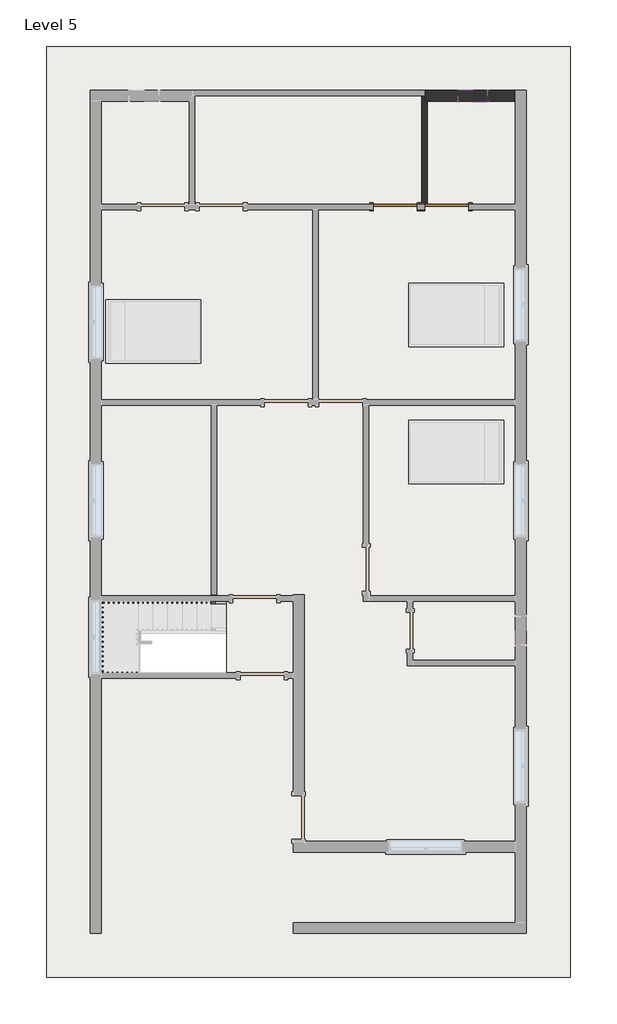
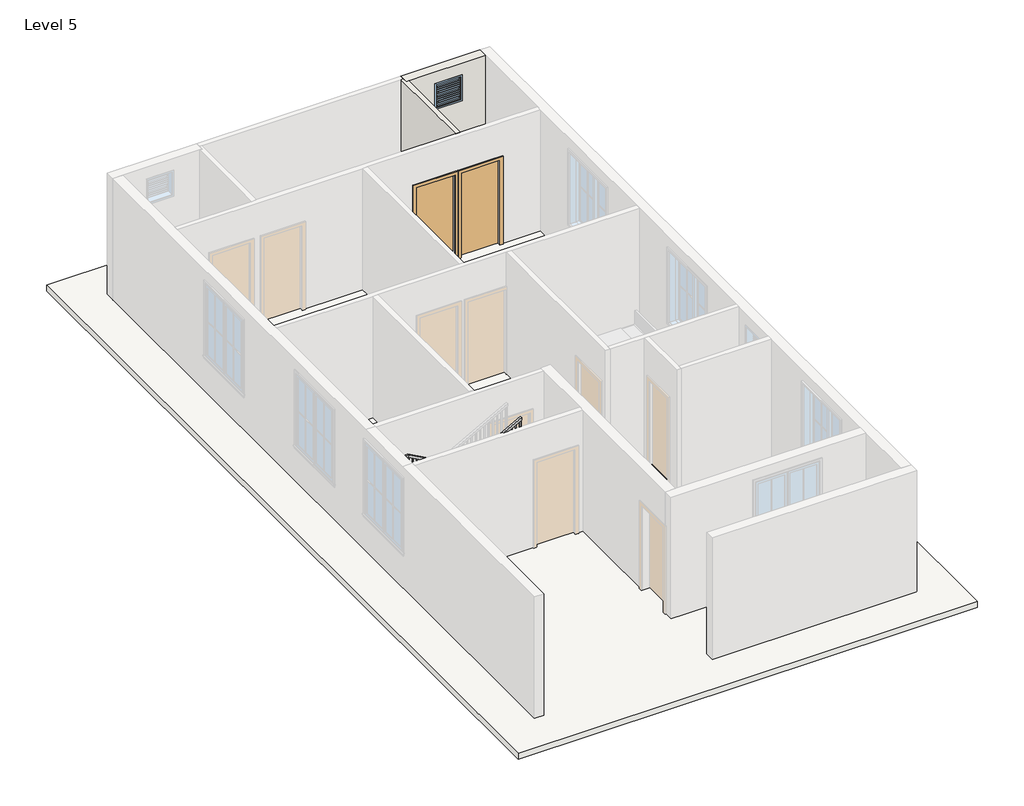
# One storey, part 2 of 3: 2 doors, 2 walls, 1 railing, 1 roof, 1 window.
"""IFC4 building model written with IfcOpenShell, lengths in millimetres."""

from ifc_helpers import new_model, si_unit, frame, origin, place, context, project, spatial, polyline, outline, extrude, faceted_brep, transform, mapped, element, save
from components import single_flush_door_3_e5f9f3c4, single_flush_door_3_305aa2a5, window_f2d8fef0

model = new_model("IFC4")

# Units and contexts
model_context = context("Model", 3, world=origin())
ifc_project = project(units=[si_unit("LENGTHUNIT", "METRE", prefix="MILLI")], contexts=[model_context])

# Site, building, storey
site = spatial("IfcSite", under=ifc_project)
building = spatial("IfcBuilding", under=site)
storey = spatial("IfcBuildingStorey", under=building, Name="Level 5", Elevation=9601.2)

# Doors
placement = place(None, origin())
single_flush_door_3_shape = single_flush_door_3_e5f9f3c4(model_context)
element("IfcDoor", 1, ObjectType="Single-Flush : DOOR 3'", at=placement, inside=storey, context=model_context, shape_type="MappedRepresentation", body=[
    mapped(single_flush_door_3_shape, transform((555.4379845, 6040.5434309, 9601.2), x_axis=(1.0, 0.0, 0.0), y_axis=(0.0, 1.0, 0.0), z_axis=(0.0, 0.0, 1.0))),
])
single_flush_door_3_2_shape = single_flush_door_3_305aa2a5(model_context)
element("IfcDoor", 2, ObjectType="Single-Flush : DOOR 3'", at=placement, inside=storey, context=model_context, shape_type="MappedRepresentation", body=[
    mapped(single_flush_door_3_2_shape, transform((1622.2379845, 6040.5434309, 9601.2), x_axis=(-1.0, 0.0, 0.0), y_axis=(0.0, -1.0, 0.0), z_axis=(0.0, 0.0, 1.0))),
])

# Railing
element("IfcRailing", 3, ObjectType="Handrail - Rectangular", at=placement, inside=storey, context=model_context, shape_type="SolidModel", body=[
    faceted_brep([(-2968.8120155, -2220.8065691, 10684.9333333), (-2968.8120155, -2220.8065691, 10626.820221), (-2968.8120155, -2170.0065691, 10626.820221), (-2968.8120155, -2170.0065691, 10684.9333333), (-4797.6120155, -2220.8065691, 11700.9333333), (-4810.7756177, -2220.8065691, 11650.1333333), (-4810.7756177, -2170.0065691, 11650.1333333), (-4797.6120155, -2170.0065691, 11700.9333333), (-5508.8120155, -2220.8065691, 11700.9333333), (-5508.8120155, -2220.8065691, 11650.1333333), (-5559.6120155, -2170.0065691, 11650.1333333), (-5559.6120155, -2170.0065691, 11700.9333333), (-5508.8120155, -3624.1565691, 11700.9333333), (-5508.8120155, -3624.1565691, 11650.1333333), (-5559.6120155, -3674.9565691, 11650.1333333), (-5559.6120155, -3674.9565691, 11700.9333333), (-5102.4120155, -3624.1565691, 11700.9333333), (-5089.2484132, -3624.1565691, 11650.1333333), (-5089.2484132, -3674.9565691, 11650.1333333), (-5102.4120155, -3674.9565691, 11700.9333333), (-2968.8120155, -3624.1565691, 12886.2666667), (-2968.8120155, -3674.9565691, 12886.2666667), (-2968.8120155, -3674.9565691, 12828.1535543), (-2968.8120155, -3624.1565691, 12828.1535543)], [[[0, 1, 2, 3]], [[1, 0, 4, 5]], [[2, 1, 5, 6]], [[3, 2, 6, 7]], [[0, 3, 7, 4]], [[5, 4, 8, 9]], [[6, 5, 9, 10]], [[7, 6, 10, 11]], [[4, 7, 11, 8]], [[9, 8, 12, 13]], [[10, 9, 13, 14]], [[11, 10, 14, 15]], [[8, 11, 15, 12]], [[13, 12, 16, 17]], [[14, 13, 17, 18]], [[15, 14, 18, 19]], [[12, 15, 19, 16]], [[20, 21, 22, 23]], [[17, 16, 20, 23]], [[18, 17, 23, 22]], [[19, 18, 22, 21]], [[16, 19, 21, 20]]]),
    extrude(outline(polyline([(12819.3341099, -2984.6870155), (12808.7507765, -3003.7370155), (11802.5333333, -3003.7370155), (11802.5333333, -2984.6870155), (12819.3341099, -2984.6870155)])), frame((0.0, -3659.0815691, 0.0), z_axis=(0.0, 1.0, 0.0), x_axis=(0.0, 0.0, 1.0)), (0.0, 0.0, 1.0), 19.05),
    extrude(outline(polyline([(12762.8896654, -3086.2870155), (12752.3063321, -3105.3370155), (11802.5333333, -3105.3370155), (11802.5333333, -3086.2870155), (12762.8896654, -3086.2870155)])), frame((0.0, -3659.0815691, 0.0), z_axis=(0.0, 1.0, 0.0), x_axis=(0.0, 0.0, 1.0)), (0.0, 0.0, 1.0), 19.05),
    extrude(outline(polyline([(12706.445221, -3187.8870155), (12695.8618876, -3206.9370155), (11802.5333333, -3206.9370155), (11802.5333333, -3187.8870155), (12706.445221, -3187.8870155)])), frame((0.0, -3659.0815691, 0.0), z_axis=(0.0, 1.0, 0.0), x_axis=(0.0, 0.0, 1.0)), (0.0, 0.0, 1.0), 19.05),
    extrude(outline(polyline([(12650.0007765, -3289.4870155), (12639.4174432, -3308.5370155), (11633.2, -3308.5370155), (11633.2, -3289.4870155), (12650.0007765, -3289.4870155)])), frame((0.0, -3659.0815691, 0.0), z_axis=(0.0, 1.0, 0.0), x_axis=(0.0, 0.0, 1.0)), (0.0, 0.0, 1.0), 19.05),
    extrude(outline(polyline([(12593.5563321, -3391.0870155), (12582.9729988, -3410.1370155), (11633.2, -3410.1370155), (11633.2, -3391.0870155), (12593.5563321, -3391.0870155)])), frame((0.0, -3659.0815691, 0.0), z_axis=(0.0, 1.0, 0.0), x_axis=(0.0, 0.0, 1.0)), (0.0, 0.0, 1.0), 19.05),
    extrude(outline(polyline([(12537.1118876, -3492.6870155), (12526.5285543, -3511.7370155), (11633.2, -3511.7370155), (11633.2, -3492.6870155), (12537.1118876, -3492.6870155)])), frame((0.0, -3659.0815691, 0.0), z_axis=(0.0, 1.0, 0.0), x_axis=(0.0, 0.0, 1.0)), (0.0, 0.0, 1.0), 19.05),
    extrude(outline(polyline([(12480.6674432, -3594.2870155), (12470.0841099, -3613.3370155), (11463.8666667, -3613.3370155), (11463.8666667, -3594.2870155), (12480.6674432, -3594.2870155)])), frame((0.0, -3659.0815691, 0.0), z_axis=(0.0, 1.0, 0.0), x_axis=(0.0, 0.0, 1.0)), (0.0, 0.0, 1.0), 19.05),
    extrude(outline(polyline([(12424.2229988, -3695.8870155), (12413.6396654, -3714.9370155), (11463.8666667, -3714.9370155), (11463.8666667, -3695.8870155), (12424.2229988, -3695.8870155)])), frame((0.0, -3659.0815691, 0.0), z_axis=(0.0, 1.0, 0.0), x_axis=(0.0, 0.0, 1.0)), (0.0, 0.0, 1.0), 19.05),
    extrude(outline(polyline([(12367.7785543, -3797.4870155), (12357.195221, -3816.5370155), (11463.8666667, -3816.5370155), (11463.8666667, -3797.4870155), (12367.7785543, -3797.4870155)])), frame((0.0, -3659.0815691, 0.0), z_axis=(0.0, 1.0, 0.0), x_axis=(0.0, 0.0, 1.0)), (0.0, 0.0, 1.0), 19.05),
    extrude(outline(polyline([(12311.3341099, -3899.0870155), (12300.7507765, -3918.1370155), (11294.5333333, -3918.1370155), (11294.5333333, -3899.0870155), (12311.3341099, -3899.0870155)])), frame((0.0, -3659.0815691, 0.0), z_axis=(0.0, 1.0, 0.0), x_axis=(0.0, 0.0, 1.0)), (0.0, 0.0, 1.0), 19.05),
    extrude(outline(polyline([(12254.8896654, -4000.6870155), (12244.3063321, -4019.7370155), (11294.5333333, -4019.7370155), (11294.5333333, -4000.6870155), (12254.8896654, -4000.6870155)])), frame((0.0, -3659.0815691, 0.0), z_axis=(0.0, 1.0, 0.0), x_axis=(0.0, 0.0, 1.0)), (0.0, 0.0, 1.0), 19.05),
    extrude(outline(polyline([(12198.445221, -4102.2870155), (12187.8618876, -4121.3370155), (11294.5333333, -4121.3370155), (11294.5333333, -4102.2870155), (12198.445221, -4102.2870155)])), frame((0.0, -3659.0815691, 0.0), z_axis=(0.0, 1.0, 0.0), x_axis=(0.0, 0.0, 1.0)), (0.0, 0.0, 1.0), 19.05),
    extrude(outline(polyline([(12142.0007765, -4203.8870155), (12131.4174432, -4222.9370155), (11125.2, -4222.9370155), (11125.2, -4203.8870155), (12142.0007765, -4203.8870155)])), frame((0.0, -3659.0815691, 0.0), z_axis=(0.0, 1.0, 0.0), x_axis=(0.0, 0.0, 1.0)), (0.0, 0.0, 1.0), 19.05),
    extrude(outline(polyline([(12085.5563321, -4305.4870155), (12074.9729988, -4324.5370155), (11125.2, -4324.5370155), (11125.2, -4305.4870155), (12085.5563321, -4305.4870155)])), frame((0.0, -3659.0815691, 0.0), z_axis=(0.0, 1.0, 0.0), x_axis=(0.0, 0.0, 1.0)), (0.0, 0.0, 1.0), 19.05),
    extrude(outline(polyline([(12029.1118876, -4407.0870155), (12018.5285543, -4426.1370155), (11125.2, -4426.1370155), (11125.2, -4407.0870155), (12029.1118876, -4407.0870155)])), frame((0.0, -3659.0815691, 0.0), z_axis=(0.0, 1.0, 0.0), x_axis=(0.0, 0.0, 1.0)), (0.0, 0.0, 1.0), 19.05),
    extrude(outline(polyline([(11972.6674432, -4508.6870155), (11962.0841099, -4527.7370155), (10955.8666667, -4527.7370155), (10955.8666667, -4508.6870155), (11972.6674432, -4508.6870155)])), frame((0.0, -3659.0815691, 0.0), z_axis=(0.0, 1.0, 0.0), x_axis=(0.0, 0.0, 1.0)), (0.0, 0.0, 1.0), 19.05),
    extrude(outline(polyline([(11916.2229988, -4610.2870155), (11905.6396654, -4629.3370155), (10955.8666667, -4629.3370155), (10955.8666667, -4610.2870155), (11916.2229988, -4610.2870155)])), frame((0.0, -3659.0815691, 0.0), z_axis=(0.0, 1.0, 0.0), x_axis=(0.0, 0.0, 1.0)), (0.0, 0.0, 1.0), 19.05),
    extrude(outline(polyline([(11859.7785543, -4711.8870155), (11849.195221, -4730.9370155), (10955.8666667, -4730.9370155), (10955.8666667, -4711.8870155), (11859.7785543, -4711.8870155)])), frame((0.0, -3659.0815691, 0.0), z_axis=(0.0, 1.0, 0.0), x_axis=(0.0, 0.0, 1.0)), (0.0, 0.0, 1.0), 19.05),
    extrude(outline(polyline([(11803.3341099, -4813.4870155), (11792.7507765, -4832.5370155), (10786.5333333, -4832.5370155), (10786.5333333, -4813.4870155), (11803.3341099, -4813.4870155)])), frame((0.0, -3659.0815691, 0.0), z_axis=(0.0, 1.0, 0.0), x_axis=(0.0, 0.0, 1.0)), (0.0, 0.0, 1.0), 19.05),
    extrude(outline(polyline([(11746.8896654, -4915.0870155), (11736.3063321, -4934.1370155), (10786.5333333, -4934.1370155), (10786.5333333, -4915.0870155), (11746.8896654, -4915.0870155)])), frame((0.0, -3659.0815691, 0.0), z_axis=(0.0, 1.0, 0.0), x_axis=(0.0, 0.0, 1.0)), (0.0, 0.0, 1.0), 19.05),
    extrude(outline(polyline([(11690.445221, -5016.6870155), (11679.8618876, -5035.7370155), (10786.5333333, -5035.7370155), (10786.5333333, -5016.6870155), (11690.445221, -5016.6870155)])), frame((0.0, -3659.0815691, 0.0), z_axis=(0.0, 1.0, 0.0), x_axis=(0.0, 0.0, 1.0)), (0.0, 0.0, 1.0), 19.05),
    extrude(outline(polyline([(-5137.3370155, -3659.0815691), (-5137.3370155, -3640.0315691), (-5118.2870155, -3640.0315691), (-5118.2870155, -3659.0815691), (-5137.3370155, -3659.0815691)])), frame((0.0, 0.0, 10786.5333333), z_axis=(0.0, 0.0, 1.0), x_axis=(1.0, 0.0, 0.0)), (0.0, 0.0, 1.0), 863.6),
    extrude(outline(polyline([(-5238.9370155, -3659.0815691), (-5238.9370155, -3640.0315691), (-5219.8870155, -3640.0315691), (-5219.8870155, -3659.0815691), (-5238.9370155, -3659.0815691)])), frame((0.0, 0.0, 10786.5333333), z_axis=(0.0, 0.0, 1.0), x_axis=(1.0, 0.0, 0.0)), (0.0, 0.0, 1.0), 863.6),
    extrude(outline(polyline([(-5340.5370155, -3659.0815691), (-5340.5370155, -3640.0315691), (-5321.4870155, -3640.0315691), (-5321.4870155, -3659.0815691), (-5340.5370155, -3659.0815691)])), frame((0.0, 0.0, 10786.5333333), z_axis=(0.0, 0.0, 1.0), x_axis=(1.0, 0.0, 0.0)), (0.0, 0.0, 1.0), 863.6),
    extrude(outline(polyline([(-5442.1370155, -3659.0815691), (-5442.1370155, -3640.0315691), (-5423.0870155, -3640.0315691), (-5423.0870155, -3659.0815691), (-5442.1370155, -3659.0815691)])), frame((0.0, 0.0, 10786.5333333), z_axis=(0.0, 0.0, 1.0), x_axis=(1.0, 0.0, 0.0)), (0.0, 0.0, 1.0), 863.6),
    extrude(outline(polyline([(-5543.7370155, -3608.2815691), (-5524.6870155, -3608.2815691), (-5524.6870155, -3627.3315691), (-5543.7370155, -3627.3315691), (-5543.7370155, -3608.2815691)])), frame((0.0, 0.0, 10786.5333333), z_axis=(0.0, 0.0, 1.0), x_axis=(1.0, 0.0, 0.0)), (0.0, 0.0, 1.0), 863.6),
    extrude(outline(polyline([(-5543.7370155, -3506.6815691), (-5524.6870155, -3506.6815691), (-5524.6870155, -3525.7315691), (-5543.7370155, -3525.7315691), (-5543.7370155, -3506.6815691)])), frame((0.0, 0.0, 10786.5333333), z_axis=(0.0, 0.0, 1.0), x_axis=(1.0, 0.0, 0.0)), (0.0, 0.0, 1.0), 863.6),
    extrude(outline(polyline([(-5543.7370155, -3405.0815691), (-5524.6870155, -3405.0815691), (-5524.6870155, -3424.1315691), (-5543.7370155, -3424.1315691), (-5543.7370155, -3405.0815691)])), frame((0.0, 0.0, 10786.5333333), z_axis=(0.0, 0.0, 1.0), x_axis=(1.0, 0.0, 0.0)), (0.0, 0.0, 1.0), 863.6),
    extrude(outline(polyline([(-5543.7370155, -3303.4815691), (-5524.6870155, -3303.4815691), (-5524.6870155, -3322.5315691), (-5543.7370155, -3322.5315691), (-5543.7370155, -3303.4815691)])), frame((0.0, 0.0, 10786.5333333), z_axis=(0.0, 0.0, 1.0), x_axis=(1.0, 0.0, 0.0)), (0.0, 0.0, 1.0), 863.6),
    extrude(outline(polyline([(-5543.7370155, -3201.8815691), (-5524.6870155, -3201.8815691), (-5524.6870155, -3220.9315691), (-5543.7370155, -3220.9315691), (-5543.7370155, -3201.8815691)])), frame((0.0, 0.0, 10786.5333333), z_axis=(0.0, 0.0, 1.0), x_axis=(1.0, 0.0, 0.0)), (0.0, 0.0, 1.0), 863.6),
    extrude(outline(polyline([(-5543.7370155, -3100.2815691), (-5524.6870155, -3100.2815691), (-5524.6870155, -3119.3315691), (-5543.7370155, -3119.3315691), (-5543.7370155, -3100.2815691)])), frame((0.0, 0.0, 10786.5333333), z_axis=(0.0, 0.0, 1.0), x_axis=(1.0, 0.0, 0.0)), (0.0, 0.0, 1.0), 863.6),
    extrude(outline(polyline([(-5543.7370155, -2998.6815691), (-5524.6870155, -2998.6815691), (-5524.6870155, -3017.7315691), (-5543.7370155, -3017.7315691), (-5543.7370155, -2998.6815691)])), frame((0.0, 0.0, 10786.5333333), z_axis=(0.0, 0.0, 1.0), x_axis=(1.0, 0.0, 0.0)), (0.0, 0.0, 1.0), 863.6),
    extrude(outline(polyline([(-5543.7370155, -2897.0815691), (-5524.6870155, -2897.0815691), (-5524.6870155, -2916.1315691), (-5543.7370155, -2916.1315691), (-5543.7370155, -2897.0815691)])), frame((0.0, 0.0, 10786.5333333), z_axis=(0.0, 0.0, 1.0), x_axis=(1.0, 0.0, 0.0)), (0.0, 0.0, 1.0), 863.6),
    extrude(outline(polyline([(-5543.7370155, -2795.4815691), (-5524.6870155, -2795.4815691), (-5524.6870155, -2814.5315691), (-5543.7370155, -2814.5315691), (-5543.7370155, -2795.4815691)])), frame((0.0, 0.0, 10786.5333333), z_axis=(0.0, 0.0, 1.0), x_axis=(1.0, 0.0, 0.0)), (0.0, 0.0, 1.0), 863.6),
    extrude(outline(polyline([(-5543.7370155, -2693.8815691), (-5524.6870155, -2693.8815691), (-5524.6870155, -2712.9315691), (-5543.7370155, -2712.9315691), (-5543.7370155, -2693.8815691)])), frame((0.0, 0.0, 10786.5333333), z_axis=(0.0, 0.0, 1.0), x_axis=(1.0, 0.0, 0.0)), (0.0, 0.0, 1.0), 863.6),
    extrude(outline(polyline([(-5543.7370155, -2592.2815691), (-5524.6870155, -2592.2815691), (-5524.6870155, -2611.3315691), (-5543.7370155, -2611.3315691), (-5543.7370155, -2592.2815691)])), frame((0.0, 0.0, 10786.5333333), z_axis=(0.0, 0.0, 1.0), x_axis=(1.0, 0.0, 0.0)), (0.0, 0.0, 1.0), 863.6),
    extrude(outline(polyline([(-5543.7370155, -2490.6815691), (-5524.6870155, -2490.6815691), (-5524.6870155, -2509.7315691), (-5543.7370155, -2509.7315691), (-5543.7370155, -2490.6815691)])), frame((0.0, 0.0, 10786.5333333), z_axis=(0.0, 0.0, 1.0), x_axis=(1.0, 0.0, 0.0)), (0.0, 0.0, 1.0), 863.6),
    extrude(outline(polyline([(-5543.7370155, -2389.0815691), (-5524.6870155, -2389.0815691), (-5524.6870155, -2408.1315691), (-5543.7370155, -2408.1315691), (-5543.7370155, -2389.0815691)])), frame((0.0, 0.0, 10786.5333333), z_axis=(0.0, 0.0, 1.0), x_axis=(1.0, 0.0, 0.0)), (0.0, 0.0, 1.0), 863.6),
    extrude(outline(polyline([(-5543.7370155, -2287.4815691), (-5524.6870155, -2287.4815691), (-5524.6870155, -2306.5315691), (-5543.7370155, -2306.5315691), (-5543.7370155, -2287.4815691)])), frame((0.0, 0.0, 10786.5333333), z_axis=(0.0, 0.0, 1.0), x_axis=(1.0, 0.0, 0.0)), (0.0, 0.0, 1.0), 863.6),
    extrude(outline(polyline([(-5499.2870155, -2185.8815691), (-5499.2870155, -2204.9315691), (-5518.3370155, -2204.9315691), (-5518.3370155, -2185.8815691), (-5499.2870155, -2185.8815691)])), frame((0.0, 0.0, 10786.5333333), z_axis=(0.0, 0.0, 1.0), x_axis=(1.0, 0.0, 0.0)), (0.0, 0.0, 1.0), 863.6),
    extrude(outline(polyline([(-5397.6870155, -2185.8815691), (-5397.6870155, -2204.9315691), (-5416.7370155, -2204.9315691), (-5416.7370155, -2185.8815691), (-5397.6870155, -2185.8815691)])), frame((0.0, 0.0, 10786.5333333), z_axis=(0.0, 0.0, 1.0), x_axis=(1.0, 0.0, 0.0)), (0.0, 0.0, 1.0), 863.6),
    extrude(outline(polyline([(-5296.0870155, -2185.8815691), (-5296.0870155, -2204.9315691), (-5315.1370155, -2204.9315691), (-5315.1370155, -2185.8815691), (-5296.0870155, -2185.8815691)])), frame((0.0, 0.0, 10786.5333333), z_axis=(0.0, 0.0, 1.0), x_axis=(1.0, 0.0, 0.0)), (0.0, 0.0, 1.0), 863.6),
    extrude(outline(polyline([(-5194.4870155, -2185.8815691), (-5194.4870155, -2204.9315691), (-5213.5370155, -2204.9315691), (-5213.5370155, -2185.8815691), (-5194.4870155, -2185.8815691)])), frame((0.0, 0.0, 10786.5333333), z_axis=(0.0, 0.0, 1.0), x_axis=(1.0, 0.0, 0.0)), (0.0, 0.0, 1.0), 863.6),
    extrude(outline(polyline([(-5092.8870155, -2185.8815691), (-5092.8870155, -2204.9315691), (-5111.9370155, -2204.9315691), (-5111.9370155, -2185.8815691), (-5092.8870155, -2185.8815691)])), frame((0.0, 0.0, 10786.5333333), z_axis=(0.0, 0.0, 1.0), x_axis=(1.0, 0.0, 0.0)), (0.0, 0.0, 1.0), 863.6),
    extrude(outline(polyline([(-4991.2870155, -2185.8815691), (-4991.2870155, -2204.9315691), (-5010.3370155, -2204.9315691), (-5010.3370155, -2185.8815691), (-4991.2870155, -2185.8815691)])), frame((0.0, 0.0, 10786.5333333), z_axis=(0.0, 0.0, 1.0), x_axis=(1.0, 0.0, 0.0)), (0.0, 0.0, 1.0), 863.6),
    extrude(outline(polyline([(-4889.6870155, -2185.8815691), (-4889.6870155, -2204.9315691), (-4908.7370155, -2204.9315691), (-4908.7370155, -2185.8815691), (-4889.6870155, -2185.8815691)])), frame((0.0, 0.0, 10786.5333333), z_axis=(0.0, 0.0, 1.0), x_axis=(1.0, 0.0, 0.0)), (0.0, 0.0, 1.0), 863.6),
    extrude(outline(polyline([(11637.5285543, -4788.0870155), (11648.1118876, -4807.1370155), (10786.5333333, -4807.1370155), (10786.5333333, -4788.0870155), (11637.5285543, -4788.0870155)])), frame((0.0, -2204.9315691, 0.0), z_axis=(0.0, 1.0, 0.0), x_axis=(0.0, 0.0, 1.0)), (0.0, 0.0, 1.0), 19.05),
    extrude(outline(polyline([(11581.0841099, -4686.4870155), (11591.6674432, -4705.5370155), (10617.2, -4705.5370155), (10617.2, -4686.4870155), (11581.0841099, -4686.4870155)])), frame((0.0, -2204.9315691, 0.0), z_axis=(0.0, 1.0, 0.0), x_axis=(0.0, 0.0, 1.0)), (0.0, 0.0, 1.0), 19.05),
    extrude(outline(polyline([(11524.6396654, -4584.8870155), (11535.2229988, -4603.9370155), (10617.2, -4603.9370155), (10617.2, -4584.8870155), (11524.6396654, -4584.8870155)])), frame((0.0, -2204.9315691, 0.0), z_axis=(0.0, 1.0, 0.0), x_axis=(0.0, 0.0, 1.0)), (0.0, 0.0, 1.0), 19.05),
    extrude(outline(polyline([(11468.195221, -4483.2870155), (11478.7785543, -4502.3370155), (10617.2, -4502.3370155), (10617.2, -4483.2870155), (11468.195221, -4483.2870155)])), frame((0.0, -2204.9315691, 0.0), z_axis=(0.0, 1.0, 0.0), x_axis=(0.0, 0.0, 1.0)), (0.0, 0.0, 1.0), 19.05),
    extrude(outline(polyline([(11411.7507765, -4381.6870155), (11422.3341099, -4400.7370155), (10447.8666667, -4400.7370155), (10447.8666667, -4381.6870155), (11411.7507765, -4381.6870155)])), frame((0.0, -2204.9315691, 0.0), z_axis=(0.0, 1.0, 0.0), x_axis=(0.0, 0.0, 1.0)), (0.0, 0.0, 1.0), 19.05),
    extrude(outline(polyline([(11355.3063321, -4280.0870155), (11365.8896654, -4299.1370155), (10447.8666667, -4299.1370155), (10447.8666667, -4280.0870155), (11355.3063321, -4280.0870155)])), frame((0.0, -2204.9315691, 0.0), z_axis=(0.0, 1.0, 0.0), x_axis=(0.0, 0.0, 1.0)), (0.0, 0.0, 1.0), 19.05),
    extrude(outline(polyline([(11298.8618876, -4178.4870155), (11309.445221, -4197.5370155), (10447.8666667, -4197.5370155), (10447.8666667, -4178.4870155), (11298.8618876, -4178.4870155)])), frame((0.0, -2204.9315691, 0.0), z_axis=(0.0, 1.0, 0.0), x_axis=(0.0, 0.0, 1.0)), (0.0, 0.0, 1.0), 19.05),
    extrude(outline(polyline([(11242.4174432, -4076.8870155), (11253.0007765, -4095.9370155), (10278.5333333, -4095.9370155), (10278.5333333, -4076.8870155), (11242.4174432, -4076.8870155)])), frame((0.0, -2204.9315691, 0.0), z_axis=(0.0, 1.0, 0.0), x_axis=(0.0, 0.0, 1.0)), (0.0, 0.0, 1.0), 19.05),
    extrude(outline(polyline([(11185.9729988, -3975.2870155), (11196.5563321, -3994.3370155), (10278.5333333, -3994.3370155), (10278.5333333, -3975.2870155), (11185.9729988, -3975.2870155)])), frame((0.0, -2204.9315691, 0.0), z_axis=(0.0, 1.0, 0.0), x_axis=(0.0, 0.0, 1.0)), (0.0, 0.0, 1.0), 19.05),
    extrude(outline(polyline([(11129.5285543, -3873.6870155), (11140.1118876, -3892.7370155), (10278.5333333, -3892.7370155), (10278.5333333, -3873.6870155), (11129.5285543, -3873.6870155)])), frame((0.0, -2204.9315691, 0.0), z_axis=(0.0, 1.0, 0.0), x_axis=(0.0, 0.0, 1.0)), (0.0, 0.0, 1.0), 19.05),
    extrude(outline(polyline([(11073.0841099, -3772.0870155), (11083.6674432, -3791.1370155), (10109.2, -3791.1370155), (10109.2, -3772.0870155), (11073.0841099, -3772.0870155)])), frame((0.0, -2204.9315691, 0.0), z_axis=(0.0, 1.0, 0.0), x_axis=(0.0, 0.0, 1.0)), (0.0, 0.0, 1.0), 19.05),
    extrude(outline(polyline([(11016.6396654, -3670.4870155), (11027.2229988, -3689.5370155), (10109.2, -3689.5370155), (10109.2, -3670.4870155), (11016.6396654, -3670.4870155)])), frame((0.0, -2204.9315691, 0.0), z_axis=(0.0, 1.0, 0.0), x_axis=(0.0, 0.0, 1.0)), (0.0, 0.0, 1.0), 19.05),
    extrude(outline(polyline([(10960.195221, -3568.8870155), (10970.7785543, -3587.9370155), (10109.2, -3587.9370155), (10109.2, -3568.8870155), (10960.195221, -3568.8870155)])), frame((0.0, -2204.9315691, 0.0), z_axis=(0.0, 1.0, 0.0), x_axis=(0.0, 0.0, 1.0)), (0.0, 0.0, 1.0), 19.05),
    extrude(outline(polyline([(10903.7507765, -3467.2870155), (10914.3341099, -3486.3370155), (9939.8666667, -3486.3370155), (9939.8666667, -3467.2870155), (10903.7507765, -3467.2870155)])), frame((0.0, -2204.9315691, 0.0), z_axis=(0.0, 1.0, 0.0), x_axis=(0.0, 0.0, 1.0)), (0.0, 0.0, 1.0), 19.05),
    extrude(outline(polyline([(10847.3063321, -3365.6870155), (10857.8896654, -3384.7370155), (9939.8666667, -3384.7370155), (9939.8666667, -3365.6870155), (10847.3063321, -3365.6870155)])), frame((0.0, -2204.9315691, 0.0), z_axis=(0.0, 1.0, 0.0), x_axis=(0.0, 0.0, 1.0)), (0.0, 0.0, 1.0), 19.05),
    extrude(outline(polyline([(10790.8618876, -3264.0870155), (10801.445221, -3283.1370155), (9939.8666667, -3283.1370155), (9939.8666667, -3264.0870155), (10790.8618876, -3264.0870155)])), frame((0.0, -2204.9315691, 0.0), z_axis=(0.0, 1.0, 0.0), x_axis=(0.0, 0.0, 1.0)), (0.0, 0.0, 1.0), 19.05),
    extrude(outline(polyline([(10734.4174432, -3162.4870155), (10745.0007765, -3181.5370155), (9770.5333333, -3181.5370155), (9770.5333333, -3162.4870155), (10734.4174432, -3162.4870155)])), frame((0.0, -2204.9315691, 0.0), z_axis=(0.0, 1.0, 0.0), x_axis=(0.0, 0.0, 1.0)), (0.0, 0.0, 1.0), 19.05),
    extrude(outline(polyline([(10677.9729988, -3060.8870155), (10688.5563321, -3079.9370155), (9770.5333333, -3079.9370155), (9770.5333333, -3060.8870155), (10677.9729988, -3060.8870155)])), frame((0.0, -2204.9315691, 0.0), z_axis=(0.0, 1.0, 0.0), x_axis=(0.0, 0.0, 1.0)), (0.0, 0.0, 1.0), 19.05),
    extrude(outline(polyline([(-5543.7370155, -3640.0315691), (-5524.6870155, -3640.0315691), (-5524.6870155, -3659.0815691), (-5543.7370155, -3659.0815691), (-5543.7370155, -3640.0315691)])), frame((0.0, 0.0, 10786.5333333), z_axis=(0.0, 0.0, 1.0), x_axis=(1.0, 0.0, 0.0)), (0.0, 0.0, 1.0), 863.6),
    extrude(outline(polyline([(-5524.6870155, -2185.8815691), (-5524.6870155, -2204.9315691), (-5543.7370155, -2204.9315691), (-5543.7370155, -2185.8815691), (-5524.6870155, -2185.8815691)])), frame((0.0, 0.0, 10786.5333333), z_axis=(0.0, 0.0, 1.0), x_axis=(1.0, 0.0, 0.0)), (0.0, 0.0, 1.0), 863.6),
    extrude(outline(polyline([(12828.1535543, -2968.8120155), (12817.570221, -2987.8620155), (11802.5333333, -2987.8620155), (11802.5333333, -2968.8120155), (12828.1535543, -2968.8120155)])), frame((0.0, -3659.0815691, 0.0), z_axis=(0.0, 1.0, 0.0), x_axis=(0.0, 0.0, 1.0)), (0.0, 0.0, 1.0), 19.05),
    extrude(outline(polyline([(10626.820221, -2968.8120155), (10637.4035543, -2987.8620155), (9770.5333333, -2987.8620155), (9770.5333333, -2968.8120155), (10626.820221, -2968.8120155)])), frame((0.0, -2204.9315691, 0.0), z_axis=(0.0, 1.0, 0.0), x_axis=(0.0, 0.0, 1.0)), (0.0, 0.0, 1.0), 19.05),
])

# Roof
element("IfcRoof", 4, ObjectType="ROOF 6\"", at=placement, inside=storey, context=model_context, shape_type="SweptSolid", body=[
    extrude(outline(polyline([(4193.9879845, 9374.2934309), (4193.9879845, -9993.2065691), (-6702.6120155, -9993.2065691), (-6702.6120155, 9374.2934309), (4193.9879845, 9374.2934309)]), holes=[polyline([(-2968.8120155, -2150.9565691), (-5788.2120155, -2150.9565691), (-5788.2120155, -3674.9565691), (-2968.8120155, -3674.9565691), (-2968.8120155, -2150.9565691)])]), frame((0.0, 0.0, 9448.8), z_axis=(0.0, 0.0, 1.0), x_axis=(1.0, 0.0, 0.0)), (0.0, 0.0, 1.0), 152.4),
])

# Walls
element("IfcWall", 5, ObjectType="WALL 4.5\"", at=placement, inside=storey, context=model_context, shape_type="SweptSolid", body=[
    extrude(outline(polyline([(1107.8879845, 6097.6934309), (1107.8879845, 8345.5934309), (1165.0379845, 8345.5934309), (1165.0379845, 8231.2934309), (1222.1879845, 8231.2934309), (1222.1879845, 6097.6934309), (1107.8879845, 6097.6934309)])), frame((0.0, 0.0, 9601.2), z_axis=(0.0, 0.0, 1.0), x_axis=(1.0, 0.0, 0.0)), (0.0, 0.0, 1.0), 3048.0),
])
element("IfcWall", 6, ObjectType="WALL 9\"", at=placement, inside=storey, context=model_context, shape_type="Brep", body=[
    faceted_brep([(3050.9879845, 8459.8934309, 9601.2), (1165.0379845, 8459.8934309, 9601.2), (1165.0379845, 8459.8934309, 12649.2), (3050.9879845, 8459.8934309, 12649.2), (2469.9629845, 8459.8934309, 12344.4), (1860.3629845, 8459.8934309, 12344.4), (1860.3629845, 8459.8934309, 11734.8), (2469.9629845, 8459.8934309, 11734.8), (3050.9879845, 8231.2934309, 9601.2), (3050.9879845, 8231.2934309, 12649.2), (1222.1879845, 8231.2934309, 12649.2), (1165.0379845, 8231.2934309, 12649.2), (1165.0379845, 8231.2934309, 9601.2), (1222.1879845, 8231.2934309, 9601.2), (2469.9629845, 8231.2934309, 12344.4), (2469.9629845, 8231.2934309, 11734.8), (1860.3629845, 8231.2934309, 11734.8), (1860.3629845, 8231.2934309, 12344.4), (1165.0379845, 8345.5934309, 9601.2), (1165.0379845, 8345.5934309, 12649.2)], [[[0, 1, 2, 3], [4, 5, 6, 7]], [[8, 9, 10, 11, 12, 13], [14, 15, 16, 17]], [[1, 0, 8, 13, 12, 18]], [[2, 1, 18, 12, 11, 19]], [[0, 3, 9, 8]], [[15, 14, 4, 7]], [[16, 15, 7, 6]], [[17, 16, 6, 5]], [[14, 17, 5, 4]], [[3, 2, 19, 11, 10, 9]]]),
])

# Window
window_shape = window_f2d8fef0(model_context)
element("IfcWindow", 7, ObjectType="Window-Louvers : 24\" x 24\"", at=placement, inside=storey, context=model_context, shape_type="MappedRepresentation", body=[
    mapped(window_shape, transform((2165.1629845, 8339.2434309, 10820.4), x_axis=(-1.0, 0.0, 0.0), y_axis=(0.0, -1.0, 0.0), z_axis=(0.0, 0.0, 1.0))),
])

save(model, "model.ifc")

# Revit data of these elements
# Type "Single-Flush : DOOR 3'"
#   Type Mark = "9"
#   Construction Type Id = "MDOOR"
#   Assembly Code = "C1020"
#   Analytic Construction = "Metal"
#   Thickness = 0' - 2"
#   Heat Transfer Coefficient (U) = 0.651978 BTU/(h·ft²·°F)
#   Height = 7' - 0"
#   Trim Projection Ext = 0' - 1"
#   Trim Projection Int = 0' - 1"
#   Trim Width = 0' - 3"
#   Width = 3' - 0"
#   Define Thermal Properties by = 1
#   Door Material = Door - Panel
#   Frame Material = Door - Frame
#   Visual Light Transmittance = 0
#   Solar Heat Gain Coefficient = 0
#   Function = (empty or 0)
#   Wall Closure = (empty or 0)
# Type "Handrail - Rectangular"
#   Assembly Code = "C2010400"
#   built-in parameter 1008612 = 0.0416667 (stored number, unit not read)
#   built-in parameter 1008611 = 0.0416667 (stored number, unit not read)
#   built-in parameter 1008609 = 0.333333 (stored number, unit not read)
#   built-in parameter 1008604 = 0.166667 (stored number, unit not read)
#   built-in parameter 1008603 = 0.166667 (stored number, unit not read)
#   Railing Height = 3' - 0"
#   built-in parameter 1008630 = 2
#   built-in parameter 1008610 = 2
#   built-in parameter 1008618 = Baluster - Square : 3/4"
# Type "ROOF 6\""
#   Assembly Code = "B1020"
#   Layers, outside or top first: 0' - 6" no material (function 1)
# Type "WALL 4.5\""
#   Assembly Code = "B2010"
#   Layers, outside or top first: 0' - 4 1/2" no material (function 1)
# Type "WALL 9\""
#   Assembly Code = "B2010"
#   Layers, outside or top first: 0' - 9" no material (function 1)
# Type "Window-Louvers : 24\" x 24\""
#   Type Mark = "19"
#   Construction Type Id = "GSP4R"
#   Assembly Code = "B20"
#   Analytic Construction = "1/8 in Pilkington single glazing"
#   Visual Light Transmittance = 0.9
#   Thermal Resistance (R) = 1.53941 (h·ft²·°F)/BTU
#   Solar Heat Gain Coefficient = 0.78
#   Max Height = 1' - 11.74264"
#   Height = 2' - 0"
#   Heat Transfer Coefficient (U) = 0.6496 BTU/(h·ft²·°F)
#   Blade Width [instance default] = 1' - 10 1/2"
#   Blade Vertical Thickness = 0' - 0.35355"
#   Blade Thickness = 0' - 0 1/4"
#   Blade Spacing = 0' - 1 1/2"
#   Blade Height = 0' - 1.85355"
#   Blade Depth = 0' - 3"
#   Blade Angle = 45.00°
#   Default Sill Height = 3' - 0"
#   Trim Projection_Exterior = 0' - 0 1/2"
#   Trim Projection_Interior = 0' - 0 1/2"
#   Trim Width_Exterior = 0' - 1 1/2"
#   Trim Width_Interior = 0' - 1 1/2"
#   Width = 2' - 0"
#   Max Blade Count = 12
#   Define Thermal Properties by = 1
#   Blade Count = 12
#   Frame Material = Birch
#   Louver Material = Birch
#   Trim Exterior Material = Birch
#   Trim Interior Material = Birch
#   Wall Closure = (empty or 0)
# Elements 1, 2 (IfcDoor, "Single-Flush : DOOR 3'")
#   Phase Created = New Construction
#   Materials on its faces: "Door - Frame", "Door - Panel"
# Element 3 (IfcRailing, "Handrail - Rectangular")
#   Phase Created = New Construction
# Element 4 (IfcRoof, "ROOF 6\"")
#   built-in parameter 1001705 = 31.5 (stored number, unit not read)
#   built-in parameter 1001701 = -0.5 (stored number, unit not read)
#   built-in parameter 1001710 = 33615
#   Phase Created = New Construction
#   Materials on its faces: "Default Roof", "Brick, Common", "Birch"
# Element 5 (IfcWall, "WALL 4.5\"")
#   Top Offset = 0' - 0"
#   Base Offset = 0' - 0"
#   Unconnected Height = 10' - 0"
#   wall height = 10' - 0"
#   Phase Created = New Construction
#   Base Constraint = Level 5
#   Materials on its faces: "Default Wall"
# Element 6 (IfcWall, "WALL 9\"")
#   Top Offset = 0' - 0"
#   Base Offset = 0' - 0"
#   Unconnected Height = 10' - 0"
#   wall height = 10' - 0"
#   Phase Created = New Construction
#   Base Constraint = Level 5
#   Materials on its faces: "Default Wall", "Brick, Common"
# Element 7 (IfcWindow, "Window-Louvers : 24\" x 24\"")
#   Mark = "39"
#   Blade Width = 1' - 10 1/2"
#   Phase Created = New Construction
#   Materials on its faces: "Birch"
# Materials
#   "Door - Panel": class "Wood", colour RGB 210 159 95, transparency 0, Cost = 0
#   "Door - Frame": colour RGB 118 70 51, transparency 0, Cost = 0
#   "Birch": class "Wood", colour RGB 224 178 126, transparency 0, Description = "Betula Alleghaniensis", Cost = 0
#   "Default Roof": colour RGB 88 101 114, transparency 0, Cost = 0
#   "Brick, Common": class "Masonry", colour RGB 170 98 104, transparency 0, Description = "Common brick", Cost = 0
#   "Default Wall": colour RGB 128 128 128, transparency 0, Cost = 0
